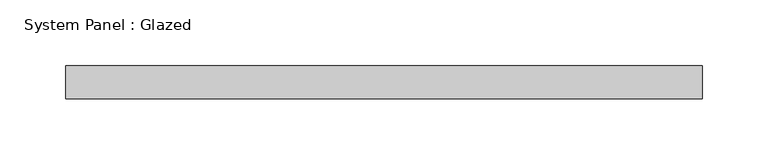
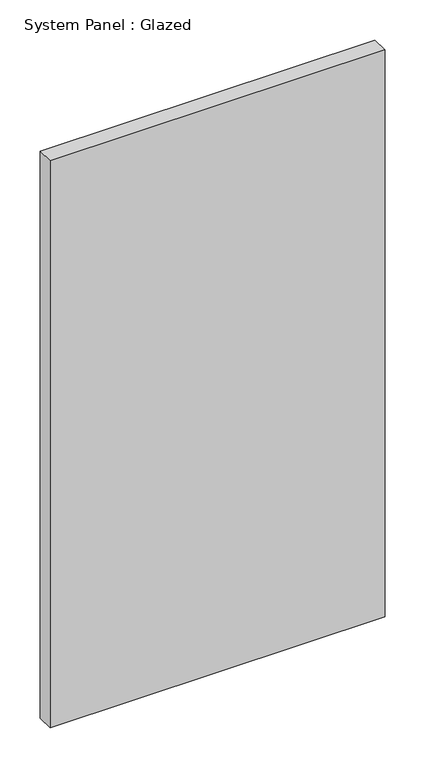
"""IFC4 building model written with IfcOpenShell, lengths in millimetres: plate geometry, System Panel : Glazed."""

from ifc_helpers import new_model, si_unit, origin, origin_with_axes, place, context, project, spatial, polyline, outline, extrude, source, transform, mapped, element, save


def system_panel_glazed_ffea3bad(model_context):
    return source(origin(), model_context, "Body", "SweptSolid", [
        extrude(outline(polyline([(241.7, 24.5), (-241.7, 24.5), (-241.7, 49.5), (241.7, 49.5), (241.7, 24.5)])), origin_with_axes(), (0.0, 0.0, 1.0), 864.4),
    ])


if __name__ == "__main__":
    model = new_model("IFC4")
    model_context = context("Model", 3, world=origin())
    ifc_project = project(units=[si_unit("LENGTHUNIT", "METRE", prefix="MILLI")], contexts=[model_context])
    site = spatial("IfcSite", under=ifc_project)
    building = spatial("IfcBuilding", under=site)
    placement = place(None, origin())
    system_panel_glazed_shape = system_panel_glazed_ffea3bad(model_context)
    element("IfcPlate", 1, ObjectType="System Panel : Glazed", at=placement, inside=building, context=model_context, shape_type="MappedRepresentation", body=[
        mapped(system_panel_glazed_shape, transform((0.0, 0.0, 0.0), x_axis=(1.0, 0.0, 0.0), y_axis=(0.0, 1.0, 0.0), z_axis=(0.0, 0.0, 1.0))),
    ])
    save(model, "model.ifc")

# Revit data of these elements
# Type "System Panel : Glazed"
#   Keynote = "H11"
#   Construction Type Id = "GSP4R"
#   Analytic Construction = "1/8 in Pilkington single glazing"
#   Visual Light Transmittance = 0.9
#   Solar Heat Gain Coefficient = 0.86
#   Heat Transfer Coefficient (U) = 6.7069 W/(m²·K)
#   Define Thermal Properties by = 1
# Element 1 (IfcPlate, "System Panel : Glazed")
#   Materials on its faces: "Glass"
# Materials
#   "Glass": class "Glass", colour RGB 0 128 192, transparency 0.9, Description = "Soda Lime Glass", Cost = 0
